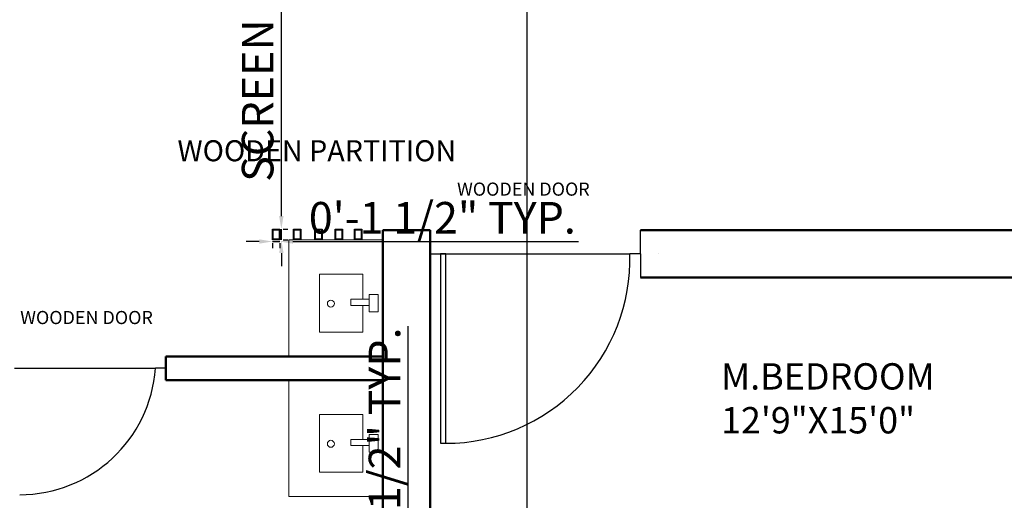
# Model space of a CAD drawing. Units: inches. Extents: x 2123 to 2977, y 1464 to 2698.
# Tile 4 of 10: x 2459 to 2647, y 2105 to 2196. Entities that reach past the tile are written whole.
import ezdxf

# ---------------------------------------------------------------- set-up
doc = ezdxf.new("R2010")
doc.units = ezdxf.units.IN
for name, color, linetype, lineweight in [('A-ANNO-DIMS', 2, 'Continuous', 18), ('A-ANNO-TEXT', 7, 'Continuous', 18), ('A-AREA-IDEN', 7, 'Continuous', 25), ('A-DOOR', 4, 'Continuous', 25), ('A-FLOR-FIXT', 8, 'Continuous', 20), ('A-WALL', 7, 'Continuous', 50), ('A-WALL-PRTN', 7, 'Continuous', 30)]:
    doc.layers.add(name, color=color, linetype=linetype, lineweight=lineweight)
doc.styles.get("Standard").update_dxf_attribs({"font": 'arial.ttf'})
doc.dimstyles.new('ISO-25', dxfattribs={"dimtxt": 6, "dimasz": 2.5, "dimexe": 1.25, "dimexo": 0.625, "dimtad": 1, "dimdec": 0, "dimlunit": 3, "dimtxsty": 'Standard', "dimcen": 2.5, "dimadec": 0, "dimazin": 0, "dimtfac": 1, "dimtdec": 0, "dimtmove": 0, "dimatfit": 3, "dimfxl": 1, "dimarcsym": 0})

# ---------------------------------------------------------------- blocks, each defined once
blk = doc.blocks.new('VANITY-BASIN')
blk.add_line((14.09, 15.62), (5.85, 15.62))
for points in [[(0, 22.13), (17.86, 22.13), (17.86, 0), (0, 0)], [(15.3, 11.79), (17.03, 11.79), (17.03, 8.46), (15.3, 8.46)]]:
    blk.add_lwpolyline(points, close=True)
for points in [[(14.09, 9.69), (14.09, 4.64), (5.85, 4.64), (5.85, 15.62)], [(14.09, 15.62), (14.09, 10.87)], [(15.3, 9.69), (11.78, 9.69), (11.78, 10.87), (15.3, 10.87)]]:
    blk.add_lwpolyline(points)
blk.add_circle((8.01, 10.03), 0.665)
blk = doc.blocks.new('TIMBER-SCREEN-UPRIGHT')
for points in [[(0, 2.02), (1.4, 2.02), (1.4, 0), (0, 0)], [(0.12, 1.92), (1.27, 1.92), (1.27, 0.12), (0.12, 0.12)]]:
    blk.add_lwpolyline(points, close=True)
blk = doc.blocks.new('*D22')
at = {"layer": 'A-ANNO-DIMS', "color": 0, "lineweight": -2, "transparency": 16777216}
for p, q in [((2509.18, 2158.53), (2509.18, 2261.23)), ((2509.18, 2154.01), (2509.18, 2156.03)), ((2509.5, 2156.03), (2510.43, 2156.03)), ((2509.5, 2154.01), (2510.43, 2154.01)), ((2509.18, 2151.51), (2509.18, 2149.01))]:
    blk.add_line(p, q, dxfattribs=at)
at = {"layer": 'A-ANNO-DIMS', "color": 0, "transparency": 16777216}
for points in [[(2508.76, 2158.53), (2509.6, 2158.53), (2509.18, 2156.03)], [(2508.76, 2151.51), (2509.6, 2151.51), (2509.18, 2154.01)]]:
    blk.add_solid(points, dxfattribs=at)
at = {"layer": 'Defpoints', "color": 0, "transparency": 16777216}
for p in [(2508.88, 2156.03), (2509.18, 2156.03), (2508.88, 2154.01)]:
    blk.add_point(p, dxfattribs=at)
at = {"layer": 'A-ANNO-DIMS', "color": 0, "transparency": 16777216, "insert": (2505.45, 2211.13), "char_height": 6, "attachment_point": 5, "rotation": 90}
blk.add_mtext('SCREEN POST 0\'-2" TYP.', dxfattribs=at)
blk = doc.blocks.new('*D23')
at = {"layer": 'A-ANNO-DIMS', "color": 0, "lineweight": -2, "transparency": 16777216}
for p, q in [((2504.98, 2153.7), (2502.48, 2153.7)), ((2507.48, 2153.7), (2508.88, 2153.7)), ((2507.48, 2153.38), (2507.48, 2152.45)), ((2508.88, 2153.38), (2508.88, 2152.45)), ((2511.38, 2153.7), (2565.68, 2153.7))]:
    blk.add_line(p, q, dxfattribs=at)
at = {"layer": 'A-ANNO-DIMS', "color": 0, "transparency": 16777216}
for points in [[(2504.98, 2154.12), (2504.98, 2153.29), (2507.48, 2153.7)], [(2511.38, 2154.12), (2511.38, 2153.29), (2508.88, 2153.7)]]:
    blk.add_solid(points, dxfattribs=at)
at = {"layer": 'Defpoints', "color": 0, "transparency": 16777216}
for p in [(2507.48, 2154.01), (2508.88, 2154.01), (2508.88, 2153.7)]:
    blk.add_point(p, dxfattribs=at)
at = {"layer": 'A-ANNO-DIMS', "color": 0, "transparency": 16777216, "insert": (2539.78, 2157.43), "char_height": 6, "attachment_point": 5}
blk.add_mtext('0\'-1 1/2" TYP.', dxfattribs=at)
blk = doc.blocks.new('*D43')
at = {"layer": 'A-ANNO-DIMS', "color": 0, "lineweight": -2, "transparency": 16777216}
for p, q in [((2533.29, 2083.88), (2533.29, 2137.62)), ((2529.06, 2083.88), (2534.54, 2083.88)), ((2533.29, 2065.8), (2533.29, 2081.38)), ((2529.06, 2063.3), (2534.54, 2063.3))]:
    blk.add_line(p, q, dxfattribs=at)
at = {"layer": 'A-ANNO-DIMS', "color": 0, "transparency": 16777216}
for points in [[(2532.87, 2081.38), (2533.71, 2081.38), (2533.29, 2083.88)], [(2532.87, 2065.8), (2533.71, 2065.8), (2533.29, 2063.3)]]:
    blk.add_solid(points, dxfattribs=at)
at = {"layer": 'Defpoints', "color": 0, "transparency": 16777216}
for p in [(2528.44, 2083.88), (2533.29, 2083.88), (2528.44, 2063.3)]:
    blk.add_point(p, dxfattribs=at)
at = {"layer": 'A-ANNO-DIMS', "color": 0, "transparency": 16777216, "insert": (2529.56, 2112), "char_height": 6, "attachment_point": 5, "rotation": 90}
blk.add_mtext('1\'-8 1/2" TYP.', dxfattribs=at)
blk = doc.blocks.new('*D57')
at = {"layer": 'A-ANNO-DIMS', "color": 0, "lineweight": -2, "transparency": 16777216}
for p, q in [((2555.89, 1805.13), (2555.89, 2606.82)), ((2558.39, 2605.57), (2755.44, 2605.57)), ((2757.94, 1805.13), (2757.94, 2606.82))]:
    blk.add_line(p, q, dxfattribs=at)
at = {"layer": 'A-ANNO-DIMS', "color": 0, "transparency": 16777216}
for points in [[(2558.39, 2605.99), (2558.39, 2605.15), (2555.89, 2605.57)], [(2755.44, 2605.99), (2755.44, 2605.15), (2757.94, 2605.57)]]:
    blk.add_solid(points, dxfattribs=at)
at = {"layer": 'Defpoints', "color": 0, "transparency": 16777216}
for p in [(2757.94, 2605.57), (2555.89, 1804.5), (2757.94, 1804.5)]:
    blk.add_point(p, dxfattribs=at)
at = {"layer": 'A-ANNO-DIMS', "color": 0, "transparency": 16777216, "insert": (2656.91, 2609.26), "char_height": 6, "attachment_point": 5}
blk.add_mtext('16\'-10"', dxfattribs=at)

msp = doc.modelspace()

# ---------------------------------------------------------------- linework, layer by layer
at = {"layer": 'A-DOOR'}
for p, q in [((2577.44, 2151.83), (2577.44, 2155.87)), ((2537.44, 2151.37), (2539.44, 2151.37)), ((2539.44, 2151.37), (2539.44, 2115.37)), ((2540.44, 2151.37), (2539.44, 2151.37)), ((2539.44, 2151.37), (2575.44, 2151.37)), ((2540.44, 2115.37), (2540.44, 2151.37)), ((2577.44, 2151.37), (2575.44, 2151.37)), ((2577.44, 2151.37), (2577.44, 2151.83)), ((2577.44, 2151.37), (2577.44, 2146.87)), ((2458.44, 2129.62), (2485.24, 2129.62)), ((2487.24, 2129.62), (2485.24, 2129.62)), ((2485.24, 2129.62), (2485.24, 2129.62)), ((2487.24, 2129.62), (2487.24, 2127.62)), ((2539.44, 2115.37), (2540.44, 2115.37))]:
    msp.add_line(p, q, dxfattribs=at)
for centre, radius, end in [((2540.44, 2150.38), 35.01, 1.6139), ((2459.44, 2131.47), 25.87, 355.9116)]:
    msp.add_arc(centre, radius, 270, end, dxfattribs=at)
at = {"layer": 'A-WALL'}
for p, q in [((2528.44, 2155.87), (2528.44, 1969.87)), ((2528.44, 2155.87), (2528.44, 1969.87)), ((2528.44, 2155.87), (2537.44, 2155.87)), ((2537.44, 2155.87), (2537.44, 1969.87)), ((2577.44, 2155.87), (2580.79, 2155.87)), ((2580.79, 2155.87), (2757.94, 2155.87)), ((2580.79, 2151.37), (2580.79, 2151.37)), ((2577.44, 2146.87), (2580.79, 2146.87)), ((2580.79, 2146.87), (2757.94, 2146.87)), ((2487.24, 2131.87), (2528.44, 2131.87)), ((2487.24, 2127.37), (2487.24, 2131.87)), ((2487.24, 2127.37), (2528.44, 2127.37))]:
    msp.add_line(p, q, dxfattribs=at)

# ---------------------------------------------------------------- block references
at = {"layer": 'A-FLOR-FIXT'}
for p in [(2510.58, 2131.87), (2510.58, 2105.24)]:
    msp.add_blockref('VANITY-BASIN', p, dxfattribs=at)
at = {"layer": 'A-WALL-PRTN'}
for p in [(2507.48, 2154.01), (2511.51, 2154.01), (2515.52, 2154.01), (2519.39, 2154.01), (2523.1, 2154.01)]:
    msp.add_blockref('TIMBER-SCREEN-UPRIGHT', p, dxfattribs=at)

# ---------------------------------------------------------------- texts
at = {"layer": 'A-ANNO-TEXT', "attachment_point": 1}
for s, width, insert, char_height in [('WOODEN PARTITION', 257.5484, (2489.43, 2172.94), 4), ('WOODEN DOOR', 84.1221, (2542.58, 2164.9), 2.5), ('WOODEN DOOR', 84.1221, (2459.54, 2140.51), 2.5)]:
    msp.add_mtext_dynamic_manual_height_columns(s, width=width, gutter_width=12.5, heights=[0], dxfattribs=dict(at, insert=insert, char_height=char_height))
at = {"layer": 'A-AREA-IDEN', "insert": (2592.76, 2130.58), "char_height": 5, "attachment_point": 1}
msp.add_mtext_dynamic_manual_height_columns('M.BEDROOM\\P12\'9"X15\'0"', width=161.7765, gutter_width=12.5, heights=[0], dxfattribs=at)

# ---------------------------------------------------------------- dimensions: what is measured, and where the dimension line sits
at = {"layer": 'A-ANNO-DIMS'}
dim = msp.add_linear_dim(base=(2757.9353, 2605.5708), p1=(2555.8869, 1804.5032), p2=(2757.9353, 1804.5032), dimstyle='ISO-25', override={"dimdec": 1, "dimlfac": 1, "dimrnd": 0, "dimzin": 1, "dimdsep": 46, "dimlunit": 4, "dimfrac": 2}, dxfattribs=at)
dim.commit()
dim.dimension.update_dxf_attribs({"geometry": '*D57', "text_midpoint": (2656.9111, 2609.2592)})
for base, p1, p2, text, picture, middle in [((2509.18, 2156.03), (2508.88, 2154.01), (2508.88, 2156.03), 'SCREEN POST <> TYP.', '*D22', (2505.45, 2211.13)), ((2533.29, 2083.88), (2528.44, 2063.3), (2528.44, 2083.88), '<> TYP.', '*D43', (2529.56, 2112))]:
    dim = msp.add_linear_dim(base=base, p1=p1, p2=p2, angle=90, text=text, dimstyle='ISO-25', override={"dimdec": 1, "dimlfac": 1, "dimrnd": 0, "dimzin": 1, "dimdsep": 46, "dimlunit": 4, "dimfrac": 2}, dxfattribs=at)
    dim.commit()
    dim.dimension.update_dxf_attribs({"geometry": picture, "text_midpoint": middle})
dim = msp.add_linear_dim(base=(2508.88, 2153.7), p1=(2507.48, 2154.01), p2=(2508.88, 2154.01), text='<> TYP.', dimstyle='ISO-25', override={"dimdec": 1, "dimlfac": 1, "dimrnd": 0, "dimzin": 1, "dimdsep": 46, "dimlunit": 4, "dimfrac": 2}, dxfattribs=at)
dim.commit()
dim.dimension.update_dxf_attribs({"geometry": '*D23', "text_midpoint": (2539.78, 2157.43)})

doc.saveas('drawing.dxf')
